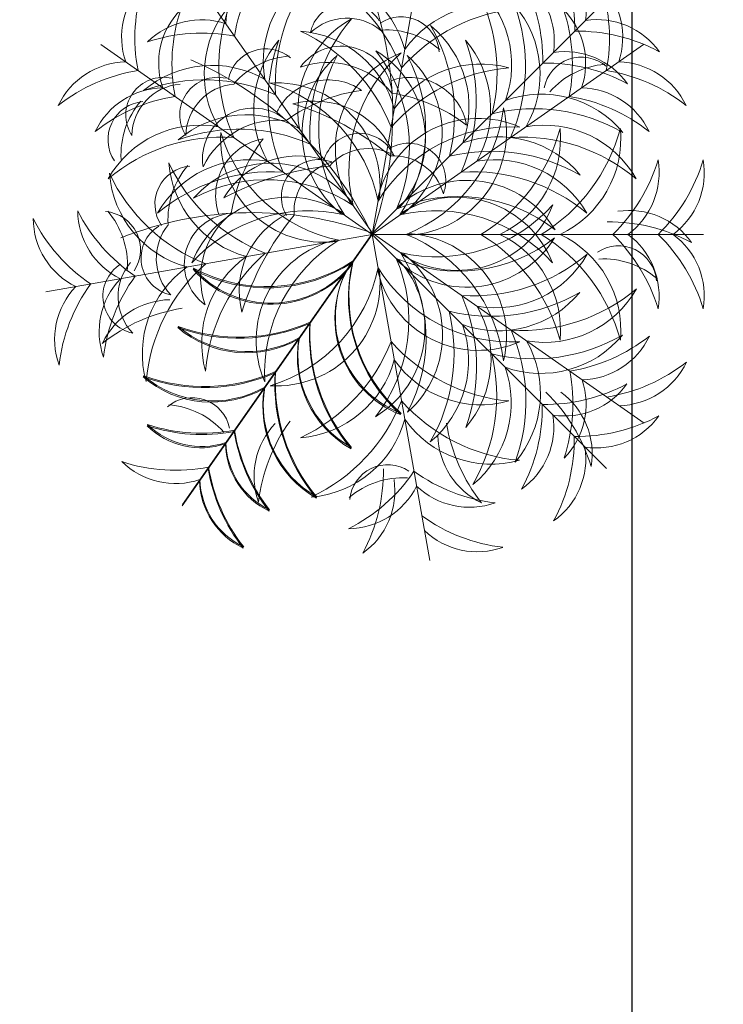
# Model space of a CAD drawing. Units: inches. Extents: x -48 to 50072, y 0 to 21068.
# Tile 29 of 75: x 440 to 467, y 289 to 327. Entities that reach past the tile are written whole.
import ezdxf

# ---------------------------------------------------------------- set-up
doc = ezdxf.new("R2010")
doc.units = ezdxf.units.IN
doc.header["$MEASUREMENT"] = 0
doc.layers.add('A-ANNO-DIMS', color=2, linetype='Continuous', lineweight=18)
doc.layers.add('L-PLNT', color=94, linetype='Continuous', lineweight=13)
doc.styles.get("Standard").update_dxf_attribs({"font": 'arial.ttf'})
doc.dimstyles.get("Standard").update_dxf_attribs({"dimtxt": 8, "dimasz": 0.18, "dimexe": 0.18, "dimexo": 0.0625, "dimgap": 0.09, "dimtad": 0, "dimtih": 1, "dimtoh": 1, "dimdec": 1, "dimzin": 0, "dimdsep": 46, "dimlunit": 4, "dimtxsty": 'Standard', "dimblk": 'ARCHTICK', "dimcen": 0.09, "dimadec": 0, "dimazin": 0, "dimtfac": 1, "dimtdec": 1, "dimtofl": 0, "dimtmove": 0, "dimatfit": 3, "dimldrblk": 'ARCHTICK', "dimfxl": 1, "dimtolj": 1, "dimtzin": 0, "dimarcsym": 0})

# ---------------------------------------------------------------- blocks, each defined once
blk = doc.blocks.new('A$C5D061C3B')
for p, q in [((3.3772, 6.6792), (3.3772, 3.3772)), ((5.2591, 6.0863), (3.3651, 3.3814)), ((1.4832, 6.082), (3.3772, 3.3772)), ((1.0302, 5.7163), (3.3651, 3.3814)), ((5.712, 5.712), (3.3772, 3.3772)), ((0.1253, 3.9506), (3.3772, 3.3772)), ((6.629, 3.9506), (3.3772, 3.3772)), ((0.6603, 1.4875), (3.3651, 3.3814)), ((1.4832, 0.6723), (3.3772, 3.3772)), ((6.0699, 1.4875), (3.3651, 3.3814)), ((3.9506, 0.1253), (3.3772, 3.3772)), ((6.082, 1.4832), (3.3772, 3.3772))]:
    blk.add_line(p, q)
for centre, radius, start, end in [((2.7629, 5.9242), 0.7621, 36.28997, 99.62433), ((2.1448, 5.0319), 1.7154, 44.07628, 73.37936), ((3.9915, 5.9242), 0.7621, 80.37567, 143.71003), ((4.6096, 5.0319), 1.7154, 106.62064, 135.92372), ((2.4194, 5.816), 0.7621, 115.37567, 178.71003), ((3.4376, 5.4395), 1.7154, 141.62064, 170.92372), ((3.9007, 5.9388), 0.7621, 125.37567, 188.71003), ((4.9688, 5.7448), 1.7154, 151.62064, 180.92372), ((3.3047, 5.4438), 1.7154, 9.07628, 38.37936), ((4.3228, 5.8202), 0.7621, 1.28997, 64.62433), ((1.9984, 5.6169), 0.7621, 125.37567, 188.71003), ((3.0665, 5.4229), 1.7154, 151.62064, 180.92372), ((2.7629, 5.4738), 0.7621, 36.28997, 99.62433), ((2.1448, 4.5814), 1.7154, 44.07628, 73.37936), ((3.9915, 5.4738), 0.7621, 80.37567, 143.71003), ((4.6096, 4.5814), 1.7154, 106.62064, 135.92372), ((3.8712, 5.8319), 0.3799, 94.742, 213.74753), ((4.4474, 5.6807), 0.826, 139.61802, 183.21064), ((4.7438, 5.6126), 0.7621, 351.28997, 54.62433), ((3.6758, 5.4187), 1.7154, 359.07628, 28.37936), ((2.6778, 5.4469), 0.7621, 115.37567, 178.71003), ((3.696, 5.0705), 1.7154, 141.62064, 170.92372), ((4.0645, 5.4512), 0.7621, 1.28997, 64.62433), ((3.0463, 5.0747), 1.7154, 9.07628, 38.37936), ((3.3438, 5.0894), 1.0556, 119.60629, 189.75109), ((4.1771, 4.8688), 1.7695, 139.96343, 183.62881), ((3.3985, 5.0936), 1.0556, 350.24891, 60.39371), ((2.5652, 4.8731), 1.7695, 356.37119, 40.03657), ((2.317, 5.2983), 0.7621, 125.37567, 188.71003), ((3.385, 5.1044), 1.7154, 151.62064, 180.92372), ((3.3573, 5.1001), 1.7154, 359.07628, 28.37936), ((4.4253, 5.2941), 0.7621, 351.28997, 54.62433), ((1.413, 5.1113), 0.7621, 71.28997, 134.62433), ((3.0349, 5.0618), 1.0556, 129.60629, 199.75109), ((3.8939, 4.9893), 1.7695, 149.96343, 193.62881), ((2.4224, 4.7989), 1.0556, 25.24891, 95.39371), ((1.8663, 4.1402), 1.7695, 31.37119, 75.03657), ((4.3319, 4.7989), 1.0556, 84.60629, 154.75109), ((4.888, 4.1402), 1.7695, 104.96343, 148.62881), ((2.8484, 4.9851), 1.7695, 346.37119, 30.03657), ((3.7074, 5.0576), 1.0556, 340.24891, 50.39371), ((1.4185, 4.0258), 1.7154, 79.07628, 108.37936), ((1.9907, 5.4623), 0.3799, 139.742, 258.74753), ((2.5051, 5.7628), 0.826, 184.61802, 228.21064), ((1.1297, 4.7481), 0.7621, 81.28997, 144.62433), ((1.6714, 4.7422), 0.7621, 71.28997, 134.62433), ((3.6883, 4.5973), 1.0556, 119.60629, 189.75109), ((4.5216, 4.3768), 1.7695, 139.96343, 183.62881), ((2.2207, 4.3811), 1.7695, 356.37119, 40.03657), ((3.054, 4.6016), 1.0556, 350.24891, 60.39371), ((5.0709, 4.7465), 0.7621, 45.37567, 108.71003), ((5.5642, 4.8068), 0.7621, 80.37567, 143.71003), ((6.1823, 3.9144), 1.7154, 106.62064, 135.92372), ((5.6126, 4.7438), 0.7621, 35.37567, 98.71003), ((3.4596, 4.6371), 1.0556, 129.60629, 199.75109), ((4.3186, 4.5646), 1.7695, 149.96343, 193.62881), ((3.2827, 4.6328), 1.0556, 340.24891, 50.39371), ((2.4237, 4.5604), 1.7695, 346.37119, 30.03657), ((1.3236, 3.68), 1.7154, 89.07628, 118.37936), ((1.6769, 3.6567), 1.7154, 79.07628, 108.37936), ((5.0653, 3.661), 1.7154, 71.62064, 100.92372), ((5.4187, 3.6758), 1.7154, 61.62064, 90.92372), ((2.4224, 4.1982), 1.0556, 25.24891, 95.39371), ((1.8663, 3.5396), 1.7695, 31.37119, 75.03657), ((4.3319, 4.1982), 1.0556, 84.60629, 154.75109), ((4.888, 3.5396), 1.7695, 104.96343, 148.62881), ((1.4482, 4.4296), 0.7621, 81.28997, 144.62433), ((3.8676, 4.3207), 1.029, 121.36542, 221.57406), ((4.5556, 4.2369), 1.5567, 141.81221, 203.33354), ((4.0352, 4.215), 1.029, 111.36542, 211.57406), ((2.7071, 4.2192), 1.029, 328.42594, 68.63458), ((2.0441, 4.0172), 1.5567, 346.66646, 48.18779), ((4.6982, 4.0129), 1.5567, 131.81221, 193.33354), ((2.1867, 4.2327), 1.5567, 336.66646, 38.18779), ((2.8746, 4.3165), 1.029, 318.42594, 58.63458), ((5.2941, 4.4253), 0.7621, 35.37567, 98.71003), ((1.6421, 3.3615), 1.7154, 89.07628, 118.37936), ((1.7796, 3.9941), 1.0556, 60.24891, 130.39371), ((4.9626, 3.9984), 1.0556, 49.60629, 119.75109), ((5.1001, 3.3573), 1.7154, 61.62064, 90.92372), ((5.0404, 3.1399), 1.7695, 69.96343, 113.62881), ((2.1429, 4.5643), 1.0556, 164.60629, 234.75109), ((1.7019, 3.1357), 1.7695, 66.37119, 110.03657), ((2.888, 4.9976), 1.7695, 184.96343, 228.62881), ((3.25, 4.4348), 1.029, 156.36542, 256.57406), ((3.8617, 4.7608), 1.5567, 176.81221, 238.33354), ((2.8927, 4.7608), 1.5567, 301.66646, 3.18779), ((3.5043, 4.4348), 1.029, 283.42594, 23.63458), ((3.8663, 4.9976), 1.7695, 311.37119, 355.03657), ((4.6115, 4.5643), 1.0556, 305.24891, 15.39371), ((1.6847, 3.7116), 1.0556, 70.24891, 140.39371), ((2.7344, 4.46), 1.0556, 164.60629, 234.75109), ((3.4796, 4.8933), 1.7695, 184.96343, 228.62881), ((2.3576, 3.686), 1.029, 3.42594, 103.63458), ((4.3967, 3.686), 1.029, 76.36542, 176.57406), ((3.2748, 4.8933), 1.7695, 311.37119, 355.03657), ((4.02, 4.46), 1.0556, 305.24891, 15.39371), ((5.0576, 3.7074), 1.0556, 39.60629, 109.75109), ((0.9755, 4.4244), 0.7621, 160.37567, 223.71003), ((1.9616, 4.8782), 1.7154, 186.62064, 215.92372), ((1.1202, 4.3101), 0.3799, 94.742, 213.74753), ((1.6965, 4.1589), 0.826, 139.61802, 183.21064), ((1.7572, 2.8527), 1.7695, 76.37119, 120.03657), ((1.9304, 3.1403), 1.5567, 21.66646, 83.18779), ((4.8239, 3.1403), 1.5567, 96.81221, 158.33354), ((4.9851, 2.8484), 1.7695, 59.96343, 103.62881), ((4.7927, 4.8782), 1.7154, 324.07628, 353.37936), ((5.7789, 4.4244), 0.7621, 316.28997, 19.62433), ((1.4191, 4.3462), 0.7621, 160.37567, 223.71003), ((2.4052, 4.8), 1.7154, 186.62064, 215.92372), ((2.1242, 3.5021), 1.0556, 60.24891, 130.39371), ((4.6181, 3.5064), 1.0556, 49.60629, 119.75109), ((4.3491, 4.8), 1.7154, 324.07628, 353.37936), ((5.3352, 4.3462), 0.7621, 316.28997, 19.62433), ((4.6959, 2.6479), 1.7695, 69.96343, 113.62881), ((4.9885, 5.8124), 1.7154, 279.07628, 308.37936), ((5.3649, 4.7942), 0.7621, 271.28997, 334.62433), ((2.1094, 3.2869), 1.0556, 70.24891, 140.39371), ((2.0464, 2.6436), 1.7695, 66.37119, 110.03657), ((4.6328, 3.2827), 1.0556, 39.60629, 109.75109), ((2.3872, 3.7525), 0.574, 99.98654, 199.40339), ((3.5988, 3.3144), 1.651, 142.57587, 170.89417), ((2.1819, 2.428), 1.7695, 76.37119, 120.03657), ((4.5604, 2.4237), 1.7695, 59.96343, 103.62881), ((1.5885, 3.6663), 0.3799, 94.742, 213.74753), ((2.1647, 3.515), 0.826, 139.61802, 183.21064), ((2.3649, 3.0454), 1.029, 38.42594, 138.63458), ((2.8402, 3.7391), 0.3717, 69.22575, 210.12788), ((3.1091, 3.5901), 0.5151, 105.43977, 183.66943), ((4.3774, 3.0496), 1.029, 41.36542, 141.57406), ((0.7621, 3.2145), 0.7621, 116.28997, 179.62433), ((1.5336, 2.4508), 1.7154, 124.07628, 153.37936), ((0.9103, 3.8754), 0.3799, 184.742, 303.74753), ((2.4258, 2.8789), 1.029, 48.42594, 148.63458), ((2.3279, 2.3533), 1.5567, 56.66646, 118.18779), ((4.4143, 2.3575), 1.5567, 61.81221, 123.33354), ((4.3165, 2.8746), 1.029, 31.36542, 131.57406), ((1.2058, 3.1363), 0.7621, 116.28997, 179.62433), ((1.9772, 2.3726), 1.7154, 124.07628, 153.37936), ((1.0616, 4.4517), 0.826, 229.61802, 273.21064), ((2.5096, 2.1909), 1.5567, 66.66646, 128.18779), ((4.2327, 2.1867), 1.5567, 51.81221, 113.33354), ((6.0526, 3.5327), 0.3799, 146.25247, 265.258), ((4.7771, 2.3726), 1.7154, 26.62064, 55.92372), ((6.6289, 3.6839), 0.826, 176.78936, 220.38198), ((5.5486, 3.1363), 0.7621, 0.37567, 63.71003), ((1.8113, 2.6838), 1.0556, 105.24891, 175.39371), ((2.3633, 2.0218), 1.7695, 111.37119, 155.03657), ((2.7293, 4.7024), 1.5567, 221.81221, 283.33354), ((2.5273, 4.0394), 1.029, 201.36542, 301.57406), ((4.0009, 4.7024), 1.5567, 256.66646, 318.18779), ((4.0129, 4.6982), 1.5567, 256.66646, 318.18779), ((4.2029, 4.0394), 1.029, 238.42594, 338.63458), ((4.215, 4.0352), 1.029, 238.42594, 338.63458), ((4.391, 2.0218), 1.7695, 24.96343, 68.62881), ((4.9431, 2.6838), 1.0556, 4.60629, 74.75109), ((2.1851, 0.015), 3.5672, 70.47721, 111.6585), ((2.4028, 2.5795), 1.0556, 105.24891, 175.39371), ((2.9548, 1.9175), 1.7695, 111.37119, 155.03657), ((2.0067, 3.0714), 0.5057, 93.87442, 233.97626), ((2.4891, 2.9324), 0.8252, 128.75364, 199.09705), ((2.9034, 2.8005), 0.8553, 116.44767, 194.36723), ((4.7443, 1.7792), 2.7893, 140.40074, 163.13904), ((2.7415, 3.2534), 0.3717, 114.22575, 255.12788), ((3.0371, 3.3382), 0.5151, 150.43977, 228.66943), ((3.7995, 1.9175), 1.7695, 24.96343, 68.62881), ((4.3515, 2.5795), 1.0556, 4.60629, 74.75109), ((5.9345, 2.8416), 0.7621, 35.37567, 98.71003), ((1.4473, 3.129), 0.3765, 122.05775, 257.85325), ((1.7505, 3.1258), 0.5286, 140.18449, 223.65396), ((2.896, 2.4268), 1.029, 83.42594, 183.63458), ((3.3592, 1.9113), 1.5567, 101.66646, 163.18779), ((3.3951, 1.9113), 1.5567, 16.81221, 78.33354), ((3.8584, 2.4268), 1.029, 356.36542, 96.57406), ((5.7406, 1.7735), 1.7154, 61.62064, 90.92372), ((4.9116, 0.1568), 3.5672, 115.47721, 156.6585), ((6.7273, 2.1893), 3.5672, 160.47721, 201.6585), ((2.4118, 2.9425), 0.574, 144.98654, 244.40339), ((3.5783, 3.4895), 1.651, 187.57587, 215.89417), ((2.1449, 3.6925), 1.0556, 209.60629, 279.75109), ((2.3655, 4.5259), 1.7695, 229.96343, 273.62881), ((3.6969, 2.3691), 1.029, 128.42594, 228.63458), ((4.389, 2.3322), 1.5567, 146.66646, 208.18779), ((2.3412, 2.3322), 1.5567, 331.81221, 33.33354), ((2.3533, 2.3279), 1.5567, 331.81221, 33.33354), ((3.0333, 2.3691), 1.029, 311.36542, 51.57406), ((3.0454, 2.3649), 1.029, 311.36542, 51.57406), ((4.3647, 4.5259), 1.7695, 266.37119, 310.03657), ((4.3768, 4.5216), 1.7695, 266.37119, 310.03657), ((4.5853, 3.6925), 1.0556, 260.24891, 330.39371), ((4.5973, 3.6883), 1.0556, 260.24891, 330.39371), ((1.0668, 2.7485), 0.3765, 122.05775, 257.85325), ((1.3701, 2.7454), 0.5286, 140.18449, 223.65396), ((2.3279, 4.401), 1.5567, 241.81221, 303.33354), ((2.3649, 3.7089), 1.029, 221.36542, 321.57406), ((1.9113, 3.3592), 1.5567, 286.81221, 348.33354), ((4.0352, 2.5394), 1.029, 148.42594, 248.63458), ((4.6982, 2.7414), 1.5567, 166.66646, 228.18779), ((4.7608, 3.8617), 1.5567, 211.66646, 273.18779), ((2.4268, 2.896), 1.029, 266.36542, 6.57406), ((3.0031, 2.8444), 0.3717, 159.22575, 300.12788), ((3.1522, 3.1134), 0.5151, 195.43977, 273.66943), ((5.4738, 3.2139), 2.7893, 185.40074, 208.13904), ((4.4348, 3.25), 1.029, 193.42594, 293.63458), ((3.45, 2.6344), 0.8553, 161.44767, 239.36723), ((1.8734, 4.1813), 1.7695, 229.96343, 273.62881), ((1.6529, 3.348), 1.0556, 209.60629, 279.75109), ((4.0986, 2.0506), 1.7695, 156.37119, 200.03657), ((2.6316, 2.0506), 1.7695, 339.96343, 23.62881), ((2.6436, 2.0464), 1.7695, 339.96343, 23.62881), ((4.8568, 4.1813), 1.7695, 266.37119, 310.03657), ((4.8688, 4.1771), 1.7695, 266.37119, 310.03657), ((5.0773, 3.348), 1.0556, 260.24891, 330.39371), ((5.0894, 3.3438), 1.0556, 260.24891, 330.39371), ((1.1216, 2.4409), 0.3799, 139.742, 258.74753), ((1.636, 2.7415), 0.826, 184.61802, 228.21064), ((3.2401, 2.1284), 1.0556, 150.24891, 220.39371), ((3.4901, 2.1284), 1.0556, 319.60629, 29.75109), ((1.9079, 2.3168), 0.3799, 139.742, 258.74753), ((4.9631, 4.7486), 2.7893, 230.40074, 253.13904), ((3.5021, 2.1242), 1.0556, 319.60629, 29.75109), ((6.244, 3.9482), 1.7154, 234.07628, 263.37936), ((2.0464, 4.1107), 1.7695, 249.96343, 293.62881), ((2.4223, 2.6173), 0.826, 184.61802, 228.21064), ((2.6243, 2.1919), 0.5057, 138.87442, 278.97626), ((3.0637, 2.4347), 0.8252, 173.75364, 244.09705), ((4.5216, 2.3775), 1.7695, 176.37119, 220.03657), ((3.9418, 2.9077), 0.8553, 206.44767, 284.36723), ((2.1242, 3.2522), 1.0556, 229.60629, 299.75109), ((3.6066, 1.7061), 1.7695, 156.37119, 200.03657), ((3.1236, 1.7061), 1.7695, 339.96343, 23.62881), ((3.1357, 1.7019), 1.7695, 339.96343, 23.62881), ((5.7902, 2.9621), 0.7621, 226.28997, 289.62433), ((1.6718, 3.7002), 1.7154, 231.62064, 260.92372), ((1.2953, 2.6821), 0.7621, 205.37567, 268.71003), ((2.7481, 1.7839), 1.0556, 150.24891, 220.39371), ((3.4279, 3.6031), 1.651, 232.57587, 260.89417), ((2.9898, 2.3915), 0.574, 189.98654, 289.40339), ((3.6883, 2.157), 1.0556, 170.24891, 240.39371), ((1.9175, 2.9548), 1.7695, 294.96343, 338.62881), ((4.8933, 3.4796), 1.7695, 221.37119, 265.03657), ((3.9821, 1.7839), 1.0556, 319.60629, 29.75109), ((3.9941, 1.7796), 1.0556, 319.60629, 29.75109), ((5.0584, 3.7002), 1.7154, 279.07628, 308.37936), ((5.0705, 3.696), 1.7154, 279.07628, 308.37936), ((5.4349, 2.6821), 0.7621, 271.28997, 334.62433), ((5.4469, 2.6778), 0.7621, 271.28997, 334.62433), ((0.9263, 2.4237), 0.7621, 205.37567, 268.71003), ((1.3028, 3.4418), 1.7154, 231.62064, 260.92372), ((2.5795, 2.4028), 1.0556, 274.60629, 344.75109), ((4.46, 2.7344), 1.0556, 215.24891, 285.39371), ((5.4274, 3.4418), 1.7154, 279.07628, 308.37936), ((5.4395, 3.4376), 1.7154, 279.07628, 308.37936), ((5.8039, 2.4237), 0.7621, 271.28997, 334.62433), ((5.816, 2.4194), 0.7621, 271.28997, 334.62433), ((1.7019, 3.6187), 1.7695, 249.96343, 293.62881), ((3.0855, 1.6812), 1.7154, 169.07628, 198.37936), ((2.4047, 2.0492), 0.5286, 185.18449, 268.65396), ((4.1771, 1.8855), 1.7695, 176.37119, 220.03657), ((3.8099, 2.4933), 0.8252, 218.75364, 289.09705), ((3.6709, 2.011), 0.5057, 183.87442, 323.97626), ((3.6447, 1.6812), 1.7154, 341.62064, 10.92372), ((3.6567, 1.6769), 1.7154, 341.62064, 10.92372), ((1.7796, 2.7602), 1.0556, 229.60629, 299.75109), ((2, 1.6757), 0.7621, 161.28997, 224.62433), ((2.188, 1.837), 0.3765, 167.05775, 302.85325), ((5.3845, 1.5838), 0.3799, 101.25247, 220.258), ((5.8989, 1.2832), 0.826, 131.78936, 175.38198), ((4.7302, 1.6757), 0.7621, 315.37567, 18.71003), ((4.7422, 1.6714), 0.7621, 315.37567, 18.71003), ((3.3438, 1.665), 1.0556, 170.24891, 240.39371), ((2.7165, 1.4228), 1.7154, 169.07628, 198.37936), ((2.0218, 2.3633), 1.7695, 294.96343, 338.62881), ((4.9976, 2.888), 1.7695, 221.37119, 265.03657), ((4.0137, 1.4228), 1.7154, 341.62064, 10.92372), ((1.631, 1.4173), 0.7621, 161.28997, 224.62433), ((5.0992, 1.4173), 0.7621, 315.37567, 18.71003), ((3.2272, 2.169), 0.826, 229.61802, 273.21064), ((3.076, 1.5927), 0.3799, 184.742, 303.74753), ((2.6838, 1.8113), 1.0556, 274.60629, 344.75109), ((4.5643, 2.1429), 1.0556, 215.24891, 285.39371), ((5.8081, 1.7538), 1.7154, 189.07628, 218.37936), ((1.6714, 2.0121), 0.7621, 225.37567, 288.71003), ((1.6769, 3.0976), 1.7154, 251.62064, 280.92372), ((2.188, 1.299), 0.3765, 167.05775, 302.85325), ((2.4047, 1.5112), 0.5286, 185.18449, 268.65396), ((3.696, 1.6838), 1.7154, 189.07628, 218.37936), ((2.6778, 1.3074), 0.7621, 181.28997, 244.62433), ((3.6165, 1.7548), 0.5286, 230.18449, 313.65396), ((3.6133, 1.4515), 0.3765, 212.05775, 347.85325), ((4.79, 1.3774), 0.7621, 181.28997, 244.62433), ((1.4185, 2.7286), 1.7154, 251.62064, 280.92372), ((1.413, 1.6431), 0.7621, 225.37567, 288.71003), ((2.4322, 1.1245), 0.3799, 184.742, 303.74753), ((3.4376, 1.3148), 1.7154, 189.07628, 218.37936), ((2.5834, 1.7007), 0.826, 229.61802, 273.21064), ((2.3726, 1.9772), 1.7154, 296.62064, 325.92372), ((3.5285, 0.6896), 0.3799, 56.25247, 175.258), ((3.9969, 1.3743), 0.5286, 230.18449, 313.65396), ((3.9938, 1.0711), 0.3765, 212.05775, 347.85325), ((4.8, 2.4052), 1.7154, 234.07628, 263.37936), ((2.4194, 0.9384), 0.7621, 181.28997, 244.62433), ((3.6797, 0.1134), 0.826, 86.78936, 130.38198), ((3.1363, 1.2058), 0.7621, 270.37567, 333.71003), ((4.3462, 1.4191), 0.7621, 226.28997, 289.62433), ((2.4508, 1.5336), 1.7154, 296.62064, 325.92372), ((4.8782, 1.9616), 1.7154, 234.07628, 263.37936), ((3.2145, 0.7621), 0.7621, 270.37567, 333.71003), ((4.4244, 0.9755), 0.7621, 226.28997, 289.62433)]:
    blk.add_arc(centre, radius, start, end)
blk = doc.blocks.new('_ArchTick')
at = {"color": 0, "linetype": 'ByBlock', "const_width": 0.15}
blk.add_lwpolyline([(-0.5, -0.5), (0.5, 0.5)], dxfattribs=at)
blk = doc.blocks.new('*D118')
at = {"layer": 'A-ANNO-DIMS', "color": 0, "lineweight": -2, "transparency": 16777216}
for p, q in [((297.017, 488.712), (297.017, 165.945)), ((463.517, 488.712), (463.517, 165.945)), ((297.017, 166.125), (367.026, 166.125)), ((463.517, 166.125), (393.509, 166.125))]:
    blk.add_line(p, q, dxfattribs=at)
at = {"layer": 'Defpoints', "color": 0, "transparency": 16777216}
for p in [(297.017, 488.775), (463.517, 488.775), (463.517, 166.125)]:
    blk.add_point(p, dxfattribs=at)
at = {"layer": 'A-ANNO-DIMS', "color": 0, "lineweight": -2, "transparency": 16777216, "xscale": 0.18, "yscale": 0.18, "zscale": 0.18, "rotation": 180}
blk.add_blockref('_ArchTick', (297.017, 166.125), dxfattribs=at)
at = {"layer": 'A-ANNO-DIMS', "color": 0, "lineweight": -2, "transparency": 16777216, "xscale": 0.18, "yscale": 0.18, "zscale": 0.18}
blk.add_blockref('_ArchTick', (463.517, 166.125), dxfattribs=at)
at = {"layer": 'A-ANNO-DIMS', "color": 0, "transparency": 16777216, "insert": (380.267, 166.125), "char_height": 8, "attachment_point": 5}
blk.add_mtext('\\A1;166.5', dxfattribs=at)
blk = doc.blocks.new('*D119')
at = {"layer": 'A-ANNO-DIMS', "color": 0, "lineweight": -2, "transparency": 16777216}
for p, q in [((463.517, 451.012), (463.517, 165.945)), ((549.017, 451.012), (549.017, 165.945)), ((463.517, 166.125), (495.752, 166.125)), ((549.017, 166.125), (516.783, 166.125))]:
    blk.add_line(p, q, dxfattribs=at)
at = {"layer": 'Defpoints', "color": 0, "transparency": 16777216}
for p in [(463.517, 451.075), (549.017, 451.075), (549.017, 166.125)]:
    blk.add_point(p, dxfattribs=at)
at = {"layer": 'A-ANNO-DIMS', "color": 0, "lineweight": -2, "transparency": 16777216, "xscale": 0.18, "yscale": 0.18, "zscale": 0.18, "rotation": 180}
blk.add_blockref('_ArchTick', (463.517, 166.125), dxfattribs=at)
at = {"layer": 'A-ANNO-DIMS', "color": 0, "lineweight": -2, "transparency": 16777216, "xscale": 0.18, "yscale": 0.18, "zscale": 0.18}
blk.add_blockref('_ArchTick', (549.017, 166.125), dxfattribs=at)
at = {"layer": 'A-ANNO-DIMS', "color": 0, "transparency": 16777216, "insert": (506.267, 166.125), "char_height": 8, "attachment_point": 5}
blk.add_mtext('\\A1;85.5', dxfattribs=at)

msp = doc.modelspace()

# ---------------------------------------------------------------- block references
at = {"layer": 'L-PLNT', "xscale": 3.862191520948588, "yscale": 3.862191520948588, "zscale": 3.862191520948588, "rotation": 270}
msp.add_blockref('A$C5D061C3B', (440.483, 331.436), dxfattribs=at)

# ---------------------------------------------------------------- dimensions: what is measured, and where the dimension line sits
at = {"layer": 'A-ANNO-DIMS'}
for base, p1, p2, picture, middle in [((463.517, 166.125), (297.017, 488.775), (463.517, 488.775), '*D118', (380.267, 166.125)), ((549.017, 166.125), (463.517, 451.075), (549.017, 451.075), '*D119', (506.267, 166.125))]:
    dim = msp.add_linear_dim(base=base, p1=p1, p2=p2, dimstyle='Standard', override={"dimdec": 1, "dimlfac": 1, "dimrnd": 0, "dimzin": 0, "dimdsep": 46, "dimlunit": 2}, dxfattribs=at)
    dim.commit()
    dim.dimension.update_dxf_attribs({"geometry": picture, "text_midpoint": middle})

doc.saveas('drawing.dxf')
